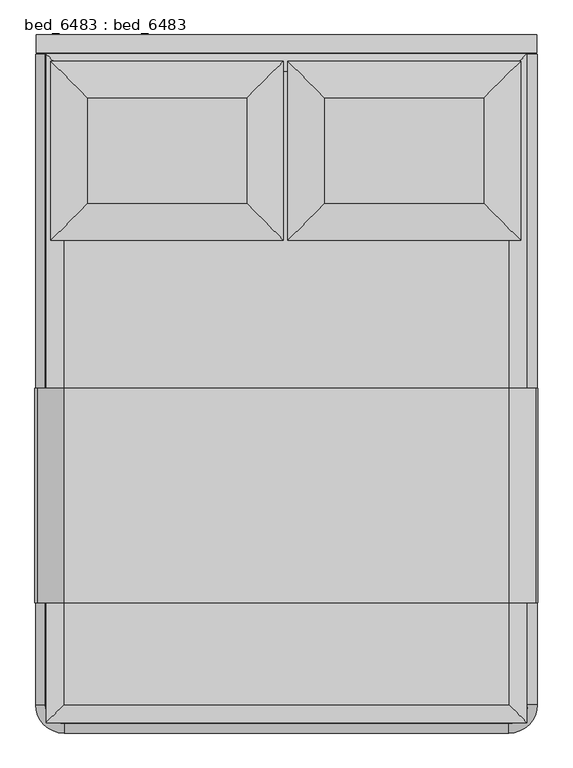
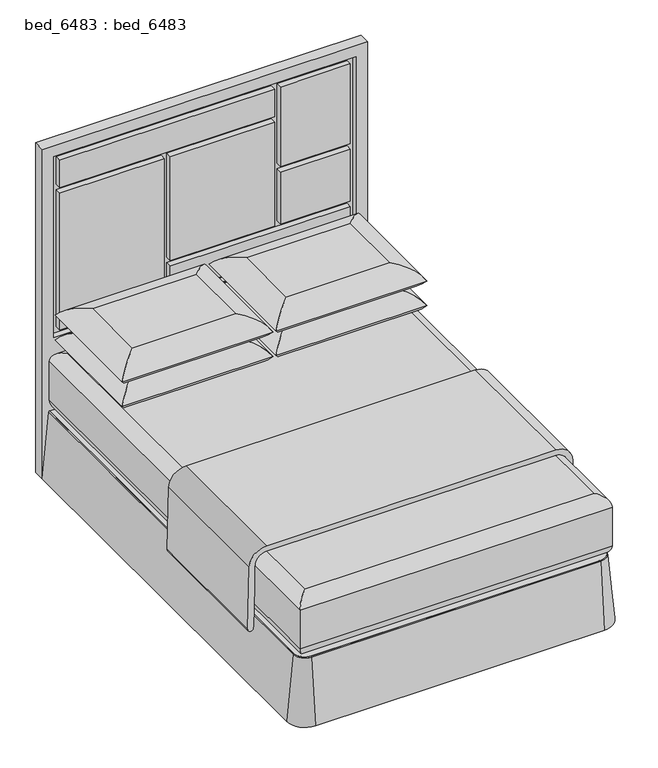
"""IFC4 building model written with IfcOpenShell, lengths in millimetres: proxy geometry, bed_6483 : bed_6483."""

from ifc_helpers import new_model, si_unit, point, frame, frame_2d, origin, place, context, project, spatial, polyline, circle_curve, ellipse_curve, trimmed, segment, composite_curve, outline, extrude, faceted_brep, source, transform, mapped, element, save
from ifc_brep_helpers import plane_surface, cylinder_surface, revolved_surface, advanced_brep


def bed_6483_bed_6483_9f93eb2d(model_context):
    return source(origin(), model_context, "Body", "SolidModel", [
        extrude(outline(composite_curve([segment(trimmed(circle_curve(frame_2d((494.8890898, 953.2998059)), 50.8), [point((494.8890898, 1004.0998059))], [point((545.6890898, 953.2998059))], False, "CARTESIAN"), True, "CONTINUOUS"), segment(polyline([(545.6890898, 953.2998059), (545.6890898, -843.7501941)]), True, "CONTINUOUS"), segment(trimmed(circle_curve(frame_2d((494.8890898, -843.7501941)), 50.8), [point((545.6890898, -843.7501941))], [point((494.8890898, -894.5501941))], False, "CARTESIAN"), True, "CONTINUOUS"), segment(polyline([(494.8890898, -894.5501941), (-768.7609102, -894.5501941)]), True, "CONTINUOUS"), segment(trimmed(circle_curve(frame_2d((-768.7609102, -843.7501941)), 50.8), [point((-768.7609102, -894.5501941))], [point((-819.5609102, -843.7501941))], False, "CARTESIAN"), True, "CONTINUOUS"), segment(polyline([(-819.5609102, -843.7501941), (-819.5609102, 953.2998059)]), True, "CONTINUOUS"), segment(trimmed(circle_curve(frame_2d((-768.7609102, 953.2998059)), 50.8), [point((-819.5609102, 953.2998059))], [point((-768.7609102, 1004.0998059))], False, "CARTESIAN"), True, "CONTINUOUS"), segment(polyline([(-768.7609102, 1004.0998059), (494.8890898, 1004.0998059)]), True, "CONTINUOUS")], self_intersect=False)), frame((0.0, 0.0, 152.4), z_axis=(0.0, 0.0, 1.0), x_axis=(1.0, 0.0, 0.0)), (0.0, 0.0, 1.0), 152.4),
        advanced_brep(
        [(-822.7359102, 1007.2748059, 149.225), (-822.7359102, 1007.2748059, 200.025), (-819.5609102, 1007.2748059, 200.025), (-819.5609102, 1007.2748059, 152.4), (-771.9359102, 1007.2748059, 152.4), (-771.9359102, 1007.2748059, 149.225), (-822.7359102, -843.7501941, 149.225), (-822.7359102, -843.7501941, 200.025), (-768.7609102, -897.7251941, 200.025), (494.8890898, -897.7251941, 200.025), (548.8640898, -843.7501941, 200.025), (548.8640898, 1007.2748059, 200.025), (545.6890898, 1007.2748059, 200.025), (545.6890898, -843.7501941, 200.025), (494.8890898, -894.5501941, 200.025), (-768.7609102, -894.5501941, 200.025), (-819.5609102, -843.7501941, 200.025), (-819.5609102, -843.7501941, 152.4), (-768.7609102, -894.5501941, 152.4), (494.8890898, -894.5501941, 152.4), (545.6890898, -843.7501941, 152.4), (545.6890898, 1007.2748059, 152.4), (498.0640898, 1007.2748059, 152.4), (498.0640898, -843.7501941, 152.4), (494.8890898, -846.9251941, 152.4), (-768.7609102, -846.9251941, 152.4), (-771.9359102, -843.7501941, 152.4), (-771.9359102, -843.7501941, 149.225), (-768.7609102, -846.9251941, 149.225), (494.8890898, -846.9251941, 149.225), (498.0640898, -843.7501941, 149.225), (498.0640898, 1007.2748059, 149.225), (548.8640898, 1007.2748059, 149.225), (548.8640898, -843.7501941, 149.225), (494.8890898, -897.7251941, 149.225), (-768.7609102, -897.7251941, 149.225)],
        [
            (0, 1),
            (1, 2),
            (2, 3),
            (3, 4),
            (4, 5),
            (5, 0),
            (0, 6),
            (6, 7),
            (7, 1),
            (7, 8, circle_curve(frame((-768.7609102, -843.7501941, 200.025), z_axis=(0.0, 0.0, 1.0), x_axis=(-1.0, 0.0, 0.0)), 53.975)),
            (8, 9),
            (9, 10, circle_curve(frame((494.8890898, -843.7501941, 200.025), z_axis=(0.0, 0.0, 1.0), x_axis=(0.0, -1.0, 0.0)), 53.975)),
            (10, 11),
            (11, 12),
            (12, 13),
            (13, 14, circle_curve(frame((494.8890898, -843.7501941, 200.025), z_axis=(0.0, 0.0, -1.0), x_axis=(0.0, -1.0, 0.0)), 50.8)),
            (14, 15),
            (15, 16, circle_curve(frame((-768.7609102, -843.7501941, 200.025), z_axis=(0.0, 0.0, -1.0), x_axis=(-1.0, 0.0, 0.0)), 50.8)),
            (16, 2),
            (16, 17),
            (17, 3),
            (17, 18, circle_curve(frame((-768.7609102, -843.7501941, 152.4), z_axis=(0.0, 0.0, 1.0), x_axis=(-1.0, 0.0, 0.0)), 50.8)),
            (18, 19),
            (19, 20, circle_curve(frame((494.8890898, -843.7501941, 152.4), z_axis=(0.0, 0.0, 1.0), x_axis=(0.0, -1.0, 0.0)), 50.8)),
            (20, 21),
            (21, 22),
            (22, 23),
            (23, 24, circle_curve(frame((494.8890898, -843.7501941, 152.4), z_axis=(0.0, 0.0, -1.0), x_axis=(0.0, -1.0, 0.0)), 3.175)),
            (24, 25),
            (25, 26, circle_curve(frame((-768.7609102, -843.7501941, 152.4), z_axis=(0.0, 0.0, -1.0), x_axis=(-1.0, 0.0, 0.0)), 3.175)),
            (26, 4),
            (26, 27),
            (27, 5),
            (27, 28, circle_curve(frame((-768.7609102, -843.7501941, 149.225), z_axis=(0.0, 0.0, 1.0), x_axis=(-1.0, 0.0, 0.0)), 3.175)),
            (28, 29),
            (29, 30, circle_curve(frame((494.8890898, -843.7501941, 149.225), z_axis=(0.0, 0.0, 1.0), x_axis=(0.0, -1.0, 0.0)), 3.175)),
            (30, 31),
            (31, 32),
            (32, 33),
            (33, 34, circle_curve(frame((494.8890898, -843.7501941, 149.225), z_axis=(0.0, 0.0, -1.0), x_axis=(0.0, -1.0, 0.0)), 53.975)),
            (34, 35),
            (35, 6, circle_curve(frame((-768.7609102, -843.7501941, 149.225), z_axis=(0.0, 0.0, -1.0), x_axis=(-1.0, 0.0, 0.0)), 53.975)),
            (35, 8),
            (15, 18),
            (25, 28),
            (34, 9),
            (14, 19),
            (24, 29),
            (33, 10),
            (13, 20),
            (23, 30),
            (31, 22),
            (21, 12),
            (11, 32),
        ],
        [
            plane_surface(frame((-822.7359102, 1007.2748059, 0.0), z_axis=(0.0, 1.0, 0.0), x_axis=(0.0, 0.0, 1.0))),
            plane_surface(frame((-822.7359102, 1007.2748059, 149.225), z_axis=(-1.0, 0.0, 0.0), x_axis=(0.0, -1.0, 0.0))),
            plane_surface(frame((-822.7359102, 1007.2748059, 200.025), z_axis=(0.0, 0.0, 1.0), x_axis=(0.0, -1.0, 0.0))),
            plane_surface(frame((-819.5609102, 1007.2748059, 200.025), z_axis=(1.0, 0.0, 0.0), x_axis=(0.0, -1.0, 0.0))),
            plane_surface(frame((-819.5609102, 1007.2748059, 152.4), z_axis=(0.0, 0.0, 1.0), x_axis=(0.0, -1.0, 0.0))),
            plane_surface(frame((-771.9359102, 1007.2748059, 152.4), z_axis=(1.0, 0.0, 0.0), x_axis=(0.0, -1.0, 0.0))),
            plane_surface(frame((-771.9359102, 1007.2748059, 149.225), z_axis=(0.0, 0.0, -1.0), x_axis=(0.0, -1.0, 0.0))),
            cylinder_surface(frame((-768.7609102, -843.7501941, 0.0), z_axis=(0.0, 0.0, 1.0), x_axis=(-1.0, 0.0, 0.0)), 53.975),
            revolved_surface(polyline([(-819.5609102, -843.7501941, 200.025), (-819.5609102, -843.7501941, 152.4)]), (-768.7609102, -843.7501941, 0.0), (0.0, 0.0, 1.0)),
            revolved_surface(polyline([(-771.9359102, -843.7501941, 152.4), (-771.9359102, -843.7501941, 149.225)]), (-768.7609102, -843.7501941, 0.0), (0.0, 0.0, 1.0)),
            plane_surface(frame((-768.7609102, -897.7251941, 149.225), z_axis=(0.0, -1.0, 0.0), x_axis=(1.0, 0.0, 0.0))),
            plane_surface(frame((-768.7609102, -894.5501941, 200.025), z_axis=(0.0, 1.0, 0.0), x_axis=(1.0, 0.0, 0.0))),
            plane_surface(frame((-768.7609102, -846.9251941, 152.4), z_axis=(0.0, 1.0, 0.0), x_axis=(1.0, 0.0, 0.0))),
            cylinder_surface(frame((494.8890898, -843.7501941, 0.0), z_axis=(0.0, 0.0, 1.0), x_axis=(0.0, -1.0, 0.0)), 53.975),
            revolved_surface(polyline([(494.8890898, -894.5501941, 200.025), (494.8890898, -894.5501941, 152.4)]), (494.8890898, -843.7501941, 0.0), (0.0, 0.0, 1.0)),
            revolved_surface(polyline([(494.8890898, -846.9251941, 152.4), (494.8890898, -846.9251941, 149.225)]), (494.8890898, -843.7501941, 0.0), (0.0, 0.0, 1.0)),
            plane_surface(frame((548.8640898, 1007.2748059, 0.0), z_axis=(0.0, 1.0, 0.0), x_axis=(0.0, 0.0, 1.0))),
            plane_surface(frame((548.8640898, -843.7501941, 149.225), z_axis=(1.0, 0.0, 0.0), x_axis=(0.0, 1.0, 0.0))),
            plane_surface(frame((545.6890898, -843.7501941, 200.025), z_axis=(-1.0, 0.0, 0.0), x_axis=(0.0, 1.0, 0.0))),
            plane_surface(frame((498.0640898, -843.7501941, 152.4), z_axis=(-1.0, 0.0, 0.0), x_axis=(0.0, 1.0, 0.0))),
        ],
        [
            (0, [[1, 2, 3, 4, 5, 6]]),
            (1, [[-1, 7, 8, 9]]),
            (2, [[-2, -9, 10, 11, 12, 13, 14, 15, 16, 17, 18, 19]]),
            (3, [[-3, -19, 20, 21]]),
            (4, [[-4, -21, 22, 23, 24, 25, 26, 27, 28, 29, 30, 31]]),
            (5, [[-5, -31, 32, 33]]),
            (6, [[-6, -33, 34, 35, 36, 37, 38, 39, 40, 41, 42, -7]]),
            (7, [[-10, -8, -42, 43]]),
            (8, [[-22, -20, -18, 44]]),
            (9, [[-34, -32, -30, 45]]),
            (10, [[-43, -41, 46, -11]]),
            (11, [[-44, -17, 47, -23]]),
            (12, [[-45, -29, 48, -35]]),
            (13, [[-12, -46, -40, 49]]),
            (14, [[-24, -47, -16, 50]]),
            (15, [[-36, -48, -28, 51]]),
            (16, [[-38, 52, -26, 53, -14, 54]]),
            (17, [[-49, -39, -54, -13]]),
            (18, [[-50, -15, -53, -25]]),
            (19, [[-51, -27, -52, -37]]),
        ],
    ),
        advanced_brep(
        [(-847.9072605, 1004.0998059, 2.4389304), (-849.5017215, 1004.0998059, 2.4389304), (-821.334659, 1004.0998059, 302.8875968), (-817.4912932, 1004.0998059, 306.3875), (-782.9739951, 1004.0998059, 306.3875), (-782.9739951, 1004.0998059, 304.8), (-819.5609102, 1004.0998059, 304.8), (-847.9072605, -843.7501941, 2.4389304), (-768.7609102, -922.8965443, 2.4389304), (494.8890898, -922.8965443, 2.4389304), (574.0354401, -843.7501941, 2.4389304), (574.0354401, 1004.0998059, 2.4389304), (575.6299011, 1004.0998059, 2.4389304), (575.6299011, -843.7501941, 2.4389304), (494.8890898, -924.4910054, 2.4389304), (-768.7609102, -924.4910054, 2.4389304), (-849.5017215, -843.7501941, 2.4389304), (-821.334659, -843.7501941, 302.8875968), (-817.4912932, -843.7501941, 306.3875), (-768.7609102, -892.480577, 306.3875), (494.8890898, -892.480577, 306.3875), (543.6194728, -843.7501941, 306.3875), (543.6194728, 1004.0998059, 306.3875), (509.1021747, 1004.0998059, 306.3875), (509.1021747, -843.7501941, 306.3875), (494.8890898, -857.9632789, 306.3875), (-768.7609102, -857.9632789, 306.3875), (-782.9739951, -843.7501941, 306.3875), (-782.9739951, -843.7501941, 304.8), (-768.7609102, -857.9632789, 304.8), (494.8890898, -857.9632789, 304.8), (509.1021747, -843.7501941, 304.8), (509.1021747, 1004.0998059, 304.8), (545.6890898, 1004.0998059, 304.8), (545.6890898, -843.7501941, 304.8), (494.8890898, -894.5501941, 304.8), (-768.7609102, -894.5501941, 304.8), (-819.5609102, -843.7501941, 304.8), (-768.7609102, -896.3239429, 302.8875968), (494.8890898, -896.3239429, 302.8875968), (547.4628387, -843.7501941, 302.8875968), (547.4628387, 1004.0998059, 302.8875968)],
        [
            (0, 1),
            (1, 2),
            (2, 3, circle_curve(frame((-817.4912932, 1004.0998059, 302.5272813), z_axis=(0.0, 1.0, 0.0), x_axis=(1.0, 0.0, 0.0)), 3.8602187)),
            (3, 4),
            (4, 5),
            (5, 6),
            (6, 0),
            (0, 7),
            (7, 8, circle_curve(frame((-768.7609102, -843.7501941, 2.4389304), z_axis=(0.0, 0.0, 1.0), x_axis=(-1.0, 0.0, 0.0)), 79.1463503)),
            (8, 9),
            (9, 10, circle_curve(frame((494.8890898, -843.7501941, 2.4389304), z_axis=(0.0, 0.0, 1.0), x_axis=(0.0, -1.0, 0.0)), 79.1463503)),
            (10, 11),
            (11, 12),
            (12, 13),
            (13, 14, circle_curve(frame((494.8890898, -843.7501941, 2.4389304), z_axis=(0.0, 0.0, -1.0), x_axis=(0.0, -1.0, 0.0)), 80.7408113)),
            (14, 15),
            (15, 16, circle_curve(frame((-768.7609102, -843.7501941, 2.4389304), z_axis=(0.0, 0.0, -1.0), x_axis=(-1.0, 0.0, 0.0)), 80.7408113)),
            (16, 1),
            (16, 17),
            (17, 2),
            (17, 18, circle_curve(frame((-817.4912932, -843.7501941, 302.5272813), z_axis=(0.0, 1.0, 0.0), x_axis=(1.0, 0.0, 0.0)), 3.8602187)),
            (18, 3),
            (18, 19, circle_curve(frame((-768.7609102, -843.7501941, 306.3875), z_axis=(0.0, 0.0, 1.0), x_axis=(-1.0, 0.0, 0.0)), 48.730383)),
            (19, 20),
            (20, 21, circle_curve(frame((494.8890898, -843.7501941, 306.3875), z_axis=(0.0, 0.0, 1.0), x_axis=(0.0, -1.0, 0.0)), 48.730383)),
            (21, 22),
            (22, 23),
            (23, 24),
            (24, 25, circle_curve(frame((494.8890898, -843.7501941, 306.3875), z_axis=(0.0, 0.0, -1.0), x_axis=(0.0, -1.0, 0.0)), 14.2130849)),
            (25, 26),
            (26, 27, circle_curve(frame((-768.7609102, -843.7501941, 306.3875), z_axis=(0.0, 0.0, -1.0), x_axis=(-1.0, 0.0, 0.0)), 14.2130849)),
            (27, 4),
            (27, 28),
            (28, 5),
            (28, 29, circle_curve(frame((-768.7609102, -843.7501941, 304.8), z_axis=(0.0, 0.0, 1.0), x_axis=(-1.0, 0.0, 0.0)), 14.2130849)),
            (29, 30),
            (30, 31, circle_curve(frame((494.8890898, -843.7501941, 304.8), z_axis=(0.0, 0.0, 1.0), x_axis=(0.0, -1.0, 0.0)), 14.2130849)),
            (31, 32),
            (32, 33),
            (33, 34),
            (34, 35, circle_curve(frame((494.8890898, -843.7501941, 304.8), z_axis=(0.0, 0.0, -1.0), x_axis=(0.0, -1.0, 0.0)), 50.8)),
            (35, 36),
            (36, 37, circle_curve(frame((-768.7609102, -843.7501941, 304.8), z_axis=(0.0, 0.0, -1.0), x_axis=(-1.0, 0.0, 0.0)), 50.8)),
            (37, 6),
            (37, 7),
            (15, 38),
            (38, 17, circle_curve(frame((-768.7609102, -843.7501941, 302.8875968), z_axis=(0.0, 0.0, -1.0), x_axis=(-1.0, 0.0, 0.0)), 52.5737489)),
            (38, 19, circle_curve(frame((-768.7609102, -892.480577, 302.5272813), z_axis=(-1.0, 0.0, 0.0), x_axis=(0.0, 1.0, 0.0)), 3.8602187)),
            (26, 29),
            (36, 8),
            (14, 39),
            (39, 38),
            (39, 20, circle_curve(frame((494.8890898, -892.480577, 302.5272813), z_axis=(-1.0, 0.0, 0.0), x_axis=(0.0, 1.0, 0.0)), 3.8602187)),
            (25, 30),
            (35, 9),
            (13, 40),
            (40, 39, circle_curve(frame((494.8890898, -843.7501941, 302.8875968), z_axis=(0.0, 0.0, -1.0), x_axis=(0.0, -1.0, 0.0)), 52.5737489)),
            (40, 21, circle_curve(frame((543.6194728, -843.7501941, 302.5272813), z_axis=(0.0, -1.0, 0.0), x_axis=(-1.0, 0.0, 0.0)), 3.8602187)),
            (24, 31),
            (34, 10),
            (11, 33),
            (32, 23),
            (22, 41, circle_curve(frame((543.6194728, 1004.0998059, 302.5272813), z_axis=(0.0, 1.0, 0.0), x_axis=(-1.0, 0.0, 0.0)), 3.8602187)),
            (41, 12),
            (41, 40),
        ],
        [
            plane_surface(frame((-819.5609102, 1004.0998059, 304.8), z_axis=(0.0, 1.0, 0.0), x_axis=(0.0, 0.0, 1.0))),
            plane_surface(frame((-847.9072605, 1004.0998059, 2.4389304), z_axis=(0.0, 0.0, -1.0), x_axis=(0.0, -1.0, 0.0))),
            plane_surface(frame((-849.5017215, 1004.0998059, 2.4389304), z_axis=(-0.9956342260592882, 0.0, 0.09334070869305766), x_axis=(0.0, -1.0, 0.0))),
            cylinder_surface(frame((-817.4912932, 1004.0998059, 302.5272813), z_axis=(0.0, 1.0, 0.0), x_axis=(1.0, 0.0, 0.0)), 3.8602187),
            plane_surface(frame((-817.4912932, 1004.0998059, 306.3875), z_axis=(0.0, 0.0, 1.0), x_axis=(0.0, -1.0, 0.0))),
            plane_surface(frame((-782.9739951, 1004.0998059, 306.3875), z_axis=(1.0, 0.0, 0.0), x_axis=(0.0, -1.0, 0.0))),
            plane_surface(frame((-782.9739951, 1004.0998059, 304.8), z_axis=(0.0, 0.0, -1.0), x_axis=(0.0, -1.0, 0.0))),
            plane_surface(frame((-819.5609102, 1004.0998059, 304.8), z_axis=(0.9956342260592882, 0.0, -0.09334070869305766), x_axis=(0.0, -1.0, 0.0))),
            revolved_surface(polyline([(-849.5017215, -843.7501941, 2.4389304), (-821.334659, -843.7501941, 302.8875968)]), (-768.7609102, -843.7501941, 304.8), (0.0, 0.0, 1.0)),
            revolved_surface(trimmed(ellipse_curve(frame((-817.4912932, -843.7501941, 302.5272813), z_axis=(0.0, 1.0, 0.0), x_axis=(1.0, 0.0, 0.0)), 3.8602187, 3.8602187), [point((-821.334659, -843.7501941, 302.8875968))], [point((-817.4912932, -843.7501941, 306.3875))], True, "CARTESIAN"), (-768.7609102, -843.7501941, 304.8), (0.0, 0.0, 1.0)),
            revolved_surface(polyline([(-782.9739951, -843.7501941, 306.3875), (-782.9739951, -843.7501941, 304.8)]), (-768.7609102, -843.7501941, 304.8), (0.0, 0.0, 1.0)),
            revolved_surface(polyline([(-819.5609102, -843.7501941, 304.8), (-847.9072605, -843.7501941, 2.4389304)]), (-768.7609102, -843.7501941, 304.8), (0.0, 0.0, 1.0)),
            plane_surface(frame((-768.7609102, -924.4910054, 2.4389304), z_axis=(0.0, -0.9956342260592882, 0.09334070869305766), x_axis=(1.0, 0.0, 0.0))),
            cylinder_surface(frame((-768.7609102, -892.480577, 302.5272813), z_axis=(-1.0, 0.0, 0.0), x_axis=(0.0, 1.0, 0.0)), 3.8602187),
            plane_surface(frame((-768.7609102, -857.9632789, 306.3875), z_axis=(0.0, 1.0, 0.0), x_axis=(1.0, 0.0, 0.0))),
            plane_surface(frame((-768.7609102, -894.5501941, 304.8), z_axis=(0.0, 0.9956342260592882, -0.09334070869305766), x_axis=(1.0, 0.0, 0.0))),
            revolved_surface(polyline([(494.8890898, -924.4910054, 2.4389304), (494.8890898, -896.3239429, 302.8875968)]), (494.8890898, -843.7501941, 304.8), (0.0, 0.0, 1.0)),
            revolved_surface(trimmed(ellipse_curve(frame((494.8890898, -892.480577, 302.5272813), z_axis=(-1.0, 0.0, 0.0), x_axis=(0.0, 1.0, 0.0)), 3.8602187, 3.8602187), [point((494.8890898, -896.3239429, 302.8875968))], [point((494.8890898, -892.480577, 306.3875))], True, "CARTESIAN"), (494.8890898, -843.7501941, 304.8), (0.0, 0.0, 1.0)),
            revolved_surface(polyline([(494.8890898, -857.963279, 306.3875), (494.8890898, -857.963279, 304.8)]), (494.8890898, -843.7501941, 304.8), (0.0, 0.0, 1.0)),
            revolved_surface(polyline([(494.8890898, -894.5501941, 304.8), (494.8890898, -922.8965443, 2.4389304)]), (494.8890898, -843.7501941, 304.8), (0.0, 0.0, 1.0)),
            plane_surface(frame((545.6890898, 1004.0998059, 304.8), z_axis=(0.0, 1.0, 0.0), x_axis=(0.0, 0.0, 1.0))),
            plane_surface(frame((575.6299011, -843.7501941, 2.4389304), z_axis=(0.9956342260592882, 0.0, 0.09334070869305766), x_axis=(0.0, 1.0, 0.0))),
            cylinder_surface(frame((543.6194728, -843.7501941, 302.5272813), z_axis=(0.0, -1.0, 0.0), x_axis=(-1.0, 0.0, 0.0)), 3.8602187),
            plane_surface(frame((509.1021747, -843.7501941, 306.3875), z_axis=(-1.0, 0.0, 0.0), x_axis=(0.0, 1.0, 0.0))),
            plane_surface(frame((545.6890898, -843.7501941, 304.8), z_axis=(-0.9956342260592882, 0.0, -0.09334070869305766), x_axis=(0.0, 1.0, 0.0))),
        ],
        [
            (0, [[1, 2, 3, 4, 5, 6, 7]]),
            (1, [[-1, 8, 9, 10, 11, 12, 13, 14, 15, 16, 17, 18]]),
            (2, [[-2, -18, 19, 20]]),
            (3, [[-3, -20, 21, 22]]),
            (4, [[-4, -22, 23, 24, 25, 26, 27, 28, 29, 30, 31, 32]]),
            (5, [[-5, -32, 33, 34]]),
            (6, [[-6, -34, 35, 36, 37, 38, 39, 40, 41, 42, 43, 44]]),
            (7, [[-7, -44, 45, -8]]),
            (8, [[-17, 46, 47, -19]]),
            (9, [[-21, -47, 48, -23]]),
            (10, [[-31, 49, -35, -33]]),
            (11, [[-9, -45, -43, 50]]),
            (12, [[-16, 51, 52, -46]]),
            (13, [[-24, -48, -52, 53]]),
            (14, [[-30, 54, -36, -49]]),
            (15, [[-10, -50, -42, 55]]),
            (16, [[-15, 56, 57, -51]]),
            (17, [[-25, -53, -57, 58]]),
            (18, [[-29, 59, -37, -54]]),
            (19, [[-11, -55, -41, 60]]),
            (20, [[-13, 61, -39, 62, -27, 63, 64]]),
            (21, [[-14, -64, 65, -56]]),
            (22, [[-26, -58, -65, -63]]),
            (23, [[-28, -62, -38, -59]]),
            (24, [[-12, -60, -40, -61]]),
        ],
    ),
        advanced_brep(
        [(-768.7609102, -843.7501941, 585.7875), (494.8890898, -843.7501941, 585.7875), (494.8890898, 470.9562082, 585.7875), (494.8890898, 953.2998059, 585.7875), (-136.9359102, 953.2998059, 585.7875), (-141.1561538, 953.2998059, 585.7875), (-768.7609102, 953.2998059, 585.7875), (-768.7609102, 470.9562082, 585.7875), (494.8890898, -843.7501941, 306.3875), (-768.7609102, -843.7501941, 306.3875), (-768.7609102, 953.2998059, 306.3875), (494.8890898, 953.2998059, 306.3875), (545.6890898, 1004.0998059, 534.9875), (545.6890898, 1004.0998059, 357.1875), (-819.5609102, 1004.0998059, 357.1875), (-819.5609102, 1004.0998059, 534.9875), (-819.5609102, -894.5501941, 357.1875), (-819.5609102, -894.5501941, 534.9875), (545.6890898, -894.5501941, 357.1875), (545.6890898, -894.5501941, 534.9875)],
        [
            (0, 1),
            (1, 2),
            (2, 3),
            (3, 4),
            (4, 5),
            (5, 6),
            (6, 7),
            (7, 0),
            (8, 9),
            (9, 10),
            (10, 11),
            (11, 8),
            (12, 13),
            (13, 14),
            (14, 15),
            (15, 12),
            (14, 16),
            (16, 17),
            (17, 15),
            (16, 18),
            (18, 19),
            (19, 17),
            (12, 19),
            (18, 13),
            (19, 1, ellipse_curve(frame((494.8890898, -843.7501941, 534.9875), z_axis=(-0.7071067811865475, -0.7071067811865475, 0.0), x_axis=(0.7071067811865476, -0.7071067811865474, 0.0)), 71.842049, 50.8)),
            (0, 17, ellipse_curve(frame((-768.7609102, -843.7501941, 534.9875), z_axis=(0.7071067811865475, -0.7071067811865475, 0.0), x_axis=(0.7071067811865476, 0.7071067811865474, 0.0)), 71.842049, 50.8)),
            (8, 18, ellipse_curve(frame((494.8890898, -843.7501941, 357.1875), z_axis=(-0.7071067811865475, -0.7071067811865475, 0.0), x_axis=(0.7071067811865476, -0.7071067811865474, 0.0)), 71.842049, 50.8)),
            (16, 9, ellipse_curve(frame((-768.7609102, -843.7501941, 357.1875), z_axis=(0.7071067811865475, -0.7071067811865475, 0.0), x_axis=(0.7071067811865476, 0.7071067811865474, 0.0)), 71.842049, 50.8)),
            (12, 3, ellipse_curve(frame((494.8890898, 953.2998059, 534.9875), z_axis=(0.7071067811865475, -0.7071067811865475, 0.0), x_axis=(0.7071067811865474, 0.7071067811865476, 0.0)), 71.842049, 50.8)),
            (11, 13, ellipse_curve(frame((494.8890898, 953.2998059, 357.1875), z_axis=(0.7071067811865475, -0.7071067811865475, 0.0), x_axis=(0.7071067811865474, 0.7071067811865476, 0.0)), 71.842049, 50.8)),
            (15, 6, ellipse_curve(frame((-768.7609102, 953.2998059, 534.9875), z_axis=(0.7071067811865475, 0.7071067811865475, 0.0), x_axis=(-0.7071067811865476, 0.7071067811865474, 0.0)), 71.842049, 50.8)),
            (10, 14, ellipse_curve(frame((-768.7609102, 953.2998059, 357.1875), z_axis=(0.7071067811865475, 0.7071067811865475, 0.0), x_axis=(-0.7071067811865476, 0.7071067811865474, 0.0)), 71.842049, 50.8)),
        ],
        [
            plane_surface(frame((-819.5609102, 1004.0998059, 585.7875), z_axis=(0.0, 0.0, 1.0), x_axis=(-1.0, 0.0, 0.0))),
            plane_surface(frame((-819.5609102, 1004.0998059, 306.3875), z_axis=(0.0, 0.0, -1.0), x_axis=(1.0, 0.0, 0.0))),
            plane_surface(frame((545.6890898, 1004.0998059, 585.7875), z_axis=(0.0, 1.0, 0.0), x_axis=(0.0, 0.0, -1.0))),
            plane_surface(frame((-819.5609102, 1004.0998059, 585.7875), z_axis=(-1.0, 0.0, 0.0), x_axis=(0.0, 0.0, -1.0))),
            plane_surface(frame((-819.5609102, -894.5501941, 585.7875), z_axis=(0.0, -1.0, 0.0), x_axis=(0.0, 0.0, -1.0))),
            plane_surface(frame((545.6890898, -894.5501941, 585.7875), z_axis=(1.0, 0.0, 0.0), x_axis=(0.0, 0.0, -1.0))),
            cylinder_surface(frame((-819.5609102, -843.7501941, 534.9875), z_axis=(1.0, 0.0, 0.0), x_axis=(0.0, 1.0, 0.0)), 50.8),
            cylinder_surface(frame((-819.5609102, -843.7501941, 357.1875), z_axis=(1.0, 0.0, 0.0), x_axis=(0.0, 1.0, 0.0)), 50.8),
            cylinder_surface(frame((494.8890898, -894.5501941, 534.9875), z_axis=(0.0, 1.0, 0.0), x_axis=(-1.0, 0.0, 0.0)), 50.8),
            cylinder_surface(frame((494.8890898, -894.5501941, 357.1875), z_axis=(0.0, 1.0, 0.0), x_axis=(-1.0, 0.0, 0.0)), 50.8),
            cylinder_surface(frame((545.6890898, 953.2998059, 534.9875), z_axis=(-1.0, 0.0, 0.0), x_axis=(0.0, -1.0, 0.0)), 50.8),
            cylinder_surface(frame((545.6890898, 953.2998059, 357.1875), z_axis=(-1.0, 0.0, 0.0), x_axis=(0.0, -1.0, 0.0)), 50.8),
            cylinder_surface(frame((-768.7609102, 1004.0998059, 534.9875), z_axis=(0.0, -1.0, 0.0), x_axis=(1.0, 0.0, 0.0)), 50.8),
            cylinder_surface(frame((-768.7609102, 1004.0998059, 357.1875), z_axis=(0.0, -1.0, 0.0), x_axis=(1.0, 0.0, 0.0)), 50.8),
        ],
        [
            (0, [[1, 2, 3, 4, 5, 6, 7, 8]]),
            (1, [[9, 10, 11, 12]]),
            (2, [[13, 14, 15, 16]]),
            (3, [[-15, 17, 18, 19]]),
            (4, [[-18, 20, 21, 22]]),
            (5, [[-13, 23, -21, 24]]),
            (6, [[25, -1, 26, -22]]),
            (7, [[27, -20, 28, -9]]),
            (8, [[-25, -23, 29, -3, -2]]),
            (9, [[-27, -12, 30, -24]]),
            (10, [[-29, -16, 31, -6, -5, -4]]),
            (11, [[-30, -11, 32, -14]]),
            (12, [[-26, -8, -7, -31, -19]]),
            (13, [[-28, -17, -32, -10]]),
        ],
    ),
        faceted_brep([(-848.1359102, 1007.2748059, 1524.0), (-848.1359102, 1007.2748059, 0.0), (-746.5359102, 1007.2748059, 0.0), (-746.5359102, 1007.2748059, 127.0), (472.6640898, 1007.2748059, 127.0), (472.6640898, 1007.2748059, 0.0), (574.2640898, 1007.2748059, 0.0), (574.2640898, 1007.2748059, 1524.0), (-797.3359102, 1007.2748059, 1473.2), (523.4640898, 1007.2748059, 1473.2), (523.4640898, 1007.2748059, 636.5875), (-797.3359102, 1007.2748059, 636.5875), (167.8640898, 1007.2748059, 1320.8), (167.8640898, 1007.2748059, 1447.8), (-771.9359102, 1007.2748059, 1447.8), (-771.9359102, 1007.2748059, 1320.8), (-314.7359102, 1007.2748059, 1295.4), (-771.9359102, 1007.2748059, 1295.4), (-771.9359102, 1007.2748059, 661.9875), (-314.7359102, 1007.2748059, 661.9875), (193.2640898, 1007.2748059, 1080.29375), (498.0640898, 1007.2748059, 1080.29375), (498.0640898, 1007.2748059, 1447.8), (193.2640898, 1007.2748059, 1447.8), (498.0640898, 1007.2748059, 1054.89375), (193.2640898, 1007.2748059, 1054.89375), (193.2640898, 1007.2748059, 814.3875), (498.0640898, 1007.2748059, 814.3875), (-289.3359102, 1007.2748059, 1295.4), (-289.3359102, 1007.2748059, 814.3875), (167.8640898, 1007.2748059, 814.3875), (167.8640898, 1007.2748059, 1295.4), (498.0640898, 1007.2748059, 661.9875), (498.0640898, 1007.2748059, 788.9875), (-289.3359102, 1007.2748059, 788.9875), (-289.3359102, 1007.2748059, 661.9875), (-848.1359102, 1058.0748059, 1524.0), (574.2640898, 1058.0748059, 1524.0), (574.2640898, 1058.0748059, 0.0), (472.6640898, 1058.0748059, 0.0), (472.6640898, 1058.0748059, 127.0), (-746.5359102, 1058.0748059, 127.0), (-746.5359102, 1058.0748059, 0.0), (-848.1359102, 1058.0748059, 0.0), (523.4640898, 1032.6748059, 1473.2), (-797.3359102, 1032.6748059, 1473.2), (-797.3359102, 1032.6748059, 636.5875), (523.4640898, 1032.6748059, 636.5875), (167.8640898, 1032.6748059, 1447.8), (167.8640898, 1032.6748059, 1320.8), (-771.9359102, 1032.6748059, 1320.8), (-771.9359102, 1032.6748059, 1447.8), (-771.9359102, 1032.6748059, 1295.4), (-314.7359102, 1032.6748059, 1295.4), (-314.7359102, 1032.6748059, 661.9875), (-771.9359102, 1032.6748059, 661.9875), (498.0640898, 1032.6748059, 1080.29375), (193.2640898, 1032.6748059, 1080.29375), (193.2640898, 1032.6748059, 1447.8), (498.0640898, 1032.6748059, 1447.8), (193.2640898, 1032.6748059, 1054.89375), (498.0640898, 1032.6748059, 1054.89375), (498.0640898, 1032.6748059, 814.3875), (193.2640898, 1032.6748059, 814.3875), (-289.3359102, 1032.6748059, 814.3875), (-289.3359102, 1032.6748059, 1295.4), (167.8640898, 1032.6748059, 1295.4), (167.8640898, 1032.6748059, 814.3875), (498.0640898, 1032.6748059, 788.9875), (498.0640898, 1032.6748059, 661.9875), (-289.3359102, 1032.6748059, 661.9875), (-289.3359102, 1032.6748059, 788.9875)], [[[0, 1, 2, 3, 4, 5, 6, 7], [8, 9, 10, 11]], [[12, 13, 14, 15]], [[16, 17, 18, 19]], [[20, 21, 22, 23]], [[24, 25, 26, 27]], [[28, 29, 30, 31]], [[32, 33, 34, 35]], [[36, 37, 38, 39, 40, 41, 42, 43]], [[1, 0, 36, 43]], [[2, 1, 43, 42]], [[3, 2, 42, 41]], [[4, 3, 41, 40]], [[5, 4, 40, 39]], [[6, 5, 39, 38]], [[7, 6, 38, 37]], [[0, 7, 37, 36]], [[44, 45, 46, 47], [48, 49, 50, 51], [52, 53, 54, 55], [56, 57, 58, 59], [60, 61, 62, 63], [64, 65, 66, 67], [68, 69, 70, 71]], [[45, 44, 9, 8]], [[46, 45, 8, 11]], [[47, 46, 11, 10]], [[44, 47, 10, 9]], [[49, 48, 13, 12]], [[50, 49, 12, 15]], [[51, 50, 15, 14]], [[48, 51, 14, 13]], [[53, 52, 17, 16]], [[54, 53, 16, 19]], [[55, 54, 19, 18]], [[52, 55, 18, 17]], [[57, 56, 21, 20]], [[58, 57, 20, 23]], [[59, 58, 23, 22]], [[56, 59, 22, 21]], [[61, 60, 25, 24]], [[62, 61, 24, 27]], [[63, 62, 27, 26]], [[60, 63, 26, 25]], [[65, 64, 29, 28]], [[66, 65, 28, 31]], [[67, 66, 31, 30]], [[64, 67, 30, 29]], [[69, 68, 33, 32]], [[70, 69, 32, 35]], [[71, 70, 35, 34]], [[68, 71, 34, 33]]]),
        advanced_brep(
        [(-28.0171423, 579.8749761, 700.0875), (423.0250783, 579.8749761, 700.0875), (423.0250783, 878.5171967, 700.0875), (-28.0171423, 878.5171967, 700.0875), (423.0250783, 579.8749761, 585.7875), (-28.0171423, 579.8749761, 585.7875), (-28.0171423, 878.5171967, 585.7875), (423.0250783, 878.5171967, 585.7875), (-132.696032, 475.1960864, 642.9375), (527.703968, 475.1960864, 642.9375), (527.703968, 983.1960864, 642.9375), (-132.696032, 983.1960864, 642.9375)],
        [
            (0, 1),
            (1, 2),
            (2, 3),
            (3, 0),
            (4, 5),
            (5, 6),
            (6, 7),
            (7, 4),
            (8, 9),
            (9, 1, ellipse_curve(frame((423.0250783, 579.8749761, 575.6448714), z_axis=(-0.7071067811865474, -0.7071067811865476, 0.0), x_axis=(0.7071067811865477, -0.7071067811865474, 0.0)), 175.9884531, 124.4426286)),
            (0, 8, ellipse_curve(frame((-28.0171423, 579.8749761, 575.6448714), z_axis=(0.7071067811865478, -0.7071067811865471, 0.0), x_axis=(0.7071067811865472, 0.7071067811865477, 0.0)), 175.9884531, 124.4426286)),
            (8, 5, ellipse_curve(frame((-28.0171423, 579.8749761, 710.2301286), z_axis=(0.7071067811865478, -0.7071067811865471, 0.0), x_axis=(0.7071067811865472, 0.7071067811865477, 0.0)), 175.9884531, 124.4426286)),
            (4, 9, ellipse_curve(frame((423.0250783, 579.8749761, 710.2301286), z_axis=(-0.7071067811865474, -0.7071067811865476, 0.0), x_axis=(0.7071067811865477, -0.7071067811865474, 0.0)), 175.9884531, 124.4426286)),
            (9, 10),
            (10, 2, ellipse_curve(frame((423.0250783, 878.5171967, 575.6448714), z_axis=(0.7071067811865476, -0.7071067811865474, 0.0), x_axis=(0.7071067811865474, 0.7071067811865478, 0.0)), 175.9884531, 124.4426286)),
            (7, 10, ellipse_curve(frame((423.0250783, 878.5171967, 710.2301286), z_axis=(0.7071067811865476, -0.7071067811865474, 0.0), x_axis=(0.7071067811865474, 0.7071067811865478, 0.0)), 175.9884531, 124.4426286)),
            (10, 11),
            (11, 3, ellipse_curve(frame((-28.0171423, 878.5171967, 575.6448714), z_axis=(0.7071067811865471, 0.7071067811865477, 0.0), x_axis=(-0.7071067811865481, 0.707106781186547, 0.0)), 175.9884531, 124.4426286)),
            (6, 11, ellipse_curve(frame((-28.0171423, 878.5171967, 710.2301286), z_axis=(0.7071067811865471, 0.7071067811865477, 0.0), x_axis=(-0.7071067811865481, 0.707106781186547, 0.0)), 175.9884531, 124.4426286)),
            (11, 8),
        ],
        [
            plane_surface(frame((-132.696032, 983.1960864, 700.0875), z_axis=(0.0, 0.0, 1.0), x_axis=(-1.0, 0.0, 0.0))),
            plane_surface(frame((-132.696032, 983.1960864, 585.7875), z_axis=(0.0, 0.0, -1.0), x_axis=(1.0, 0.0, 0.0))),
            cylinder_surface(frame((-132.696032, 579.8749761, 575.6448714), z_axis=(1.0, 0.0, 0.0), x_axis=(0.0, 1.0, 0.0)), 124.4426286),
            cylinder_surface(frame((-132.696032, 579.8749761, 710.2301286), z_axis=(1.0, 0.0, 0.0), x_axis=(0.0, 1.0, 0.0)), 124.4426286),
            cylinder_surface(frame((423.0250783, 475.1960864, 575.6448714), z_axis=(0.0, 1.0, 0.0), x_axis=(-1.0, 0.0, 0.0)), 124.4426286),
            cylinder_surface(frame((423.0250783, 475.1960864, 710.2301286), z_axis=(0.0, 1.0, 0.0), x_axis=(-1.0, 0.0, 0.0)), 124.4426286),
            cylinder_surface(frame((527.703968, 878.5171967, 575.6448714), z_axis=(-1.0, 0.0, 0.0), x_axis=(0.0, -1.0, 0.0)), 124.4426286),
            cylinder_surface(frame((527.703968, 878.5171967, 710.2301286), z_axis=(-1.0, 0.0, 0.0), x_axis=(0.0, -1.0, 0.0)), 124.4426286),
            cylinder_surface(frame((-28.0171423, 983.1960864, 575.6448714), z_axis=(0.0, -1.0, 0.0), x_axis=(1.0, 0.0, 0.0)), 124.4426286),
            cylinder_surface(frame((-28.0171423, 983.1960864, 710.2301286), z_axis=(0.0, -1.0, 0.0), x_axis=(1.0, 0.0, 0.0)), 124.4426286),
        ],
        [
            (0, [[1, 2, 3, 4]]),
            (1, [[5, 6, 7, 8]]),
            (2, [[9, 10, -1, 11]]),
            (3, [[-9, 12, -5, 13]]),
            (4, [[-10, 14, 15, -2]]),
            (5, [[-13, -8, 16, -14]]),
            (6, [[-15, 17, 18, -3]]),
            (7, [[-16, -7, 19, -17]]),
            (8, [[-11, -4, -18, 20]]),
            (9, [[-12, -20, -19, -6]]),
        ],
    ),
        advanced_brep(
        [(-701.1171423, 579.8749761, 700.0875), (-250.0749217, 579.8749761, 700.0875), (-250.0749217, 878.5171967, 700.0875), (-701.1171423, 878.5171967, 700.0875), (-250.0749217, 579.8749761, 585.7875), (-701.1171423, 579.8749761, 585.7875), (-701.1171423, 878.5171967, 585.7875), (-250.0749217, 878.5171967, 585.7875), (-805.796032, 475.1960864, 642.9375), (-145.396032, 475.1960864, 642.9375), (-145.396032, 983.1960864, 642.9375), (-805.796032, 983.1960864, 642.9375)],
        [
            (0, 1),
            (1, 2),
            (2, 3),
            (3, 0),
            (4, 5),
            (5, 6),
            (6, 7),
            (7, 4),
            (8, 9),
            (9, 1, ellipse_curve(frame((-250.0749217, 579.8749761, 575.6448714), z_axis=(-0.7071067811865475, -0.7071067811865475, 0.0), x_axis=(0.7071067811865476, -0.7071067811865475, 0.0)), 175.9884531, 124.4426286)),
            (0, 8, ellipse_curve(frame((-701.1171423, 579.8749761, 575.6448714), z_axis=(0.7071067811865477, -0.7071067811865472, 0.0), x_axis=(0.7071067811865475, 0.7071067811865475, 0.0)), 175.9884531, 124.4426286)),
            (8, 5, ellipse_curve(frame((-701.1171423, 579.8749761, 710.2301286), z_axis=(0.7071067811865477, -0.7071067811865472, 0.0), x_axis=(0.7071067811865475, 0.7071067811865475, 0.0)), 175.9884531, 124.4426286)),
            (4, 9, ellipse_curve(frame((-250.0749217, 579.8749761, 710.2301286), z_axis=(-0.7071067811865475, -0.7071067811865475, 0.0), x_axis=(0.7071067811865476, -0.7071067811865475, 0.0)), 175.9884531, 124.4426286)),
            (9, 10),
            (10, 2, ellipse_curve(frame((-250.0749217, 878.5171967, 575.6448714), z_axis=(0.7071067811865475, -0.7071067811865475, 0.0), x_axis=(0.7071067811865472, 0.7071067811865477, 0.0)), 175.9884531, 124.4426286)),
            (7, 10, ellipse_curve(frame((-250.0749217, 878.5171967, 710.2301286), z_axis=(0.7071067811865475, -0.7071067811865475, 0.0), x_axis=(0.7071067811865472, 0.7071067811865477, 0.0)), 175.9884531, 124.4426286)),
            (10, 11),
            (11, 3, ellipse_curve(frame((-701.1171423, 878.5171967, 575.6448714), z_axis=(0.7071067811865472, 0.7071067811865477, 0.0), x_axis=(-0.7071067811865478, 0.7071067811865472, 0.0)), 175.9884531, 124.4426286)),
            (6, 11, ellipse_curve(frame((-701.1171423, 878.5171967, 710.2301286), z_axis=(0.7071067811865472, 0.7071067811865477, 0.0), x_axis=(-0.7071067811865478, 0.7071067811865472, 0.0)), 175.9884531, 124.4426286)),
            (11, 8),
        ],
        [
            plane_surface(frame((-805.796032, 983.1960864, 700.0875), z_axis=(0.0, 0.0, 1.0), x_axis=(-1.0, 0.0, 0.0))),
            plane_surface(frame((-805.796032, 983.1960864, 585.7875), z_axis=(0.0, 0.0, -1.0), x_axis=(1.0, 0.0, 0.0))),
            cylinder_surface(frame((-805.796032, 579.8749761, 575.6448714), z_axis=(1.0, 0.0, 0.0), x_axis=(0.0, 1.0, 0.0)), 124.4426286),
            cylinder_surface(frame((-805.796032, 579.8749761, 710.2301286), z_axis=(1.0, 0.0, 0.0), x_axis=(0.0, 1.0, 0.0)), 124.4426286),
            cylinder_surface(frame((-250.0749217, 475.1960864, 575.6448714), z_axis=(0.0, 1.0, 0.0), x_axis=(-1.0, 0.0, 0.0)), 124.4426286),
            cylinder_surface(frame((-250.0749217, 475.1960864, 710.2301286), z_axis=(0.0, 1.0, 0.0), x_axis=(-1.0, 0.0, 0.0)), 124.4426286),
            cylinder_surface(frame((-145.396032, 878.5171967, 575.6448714), z_axis=(-1.0, 0.0, 0.0), x_axis=(0.0, -1.0, 0.0)), 124.4426286),
            cylinder_surface(frame((-145.396032, 878.5171967, 710.2301286), z_axis=(-1.0, 0.0, 0.0), x_axis=(0.0, -1.0, 0.0)), 124.4426286),
            cylinder_surface(frame((-701.1171423, 983.1960864, 575.6448714), z_axis=(0.0, -1.0, 0.0), x_axis=(1.0, 0.0, 0.0)), 124.4426286),
            cylinder_surface(frame((-701.1171423, 983.1960864, 710.2301286), z_axis=(0.0, -1.0, 0.0), x_axis=(1.0, 0.0, 0.0)), 124.4426286),
        ],
        [
            (0, [[1, 2, 3, 4]]),
            (1, [[5, 6, 7, 8]]),
            (2, [[9, 10, -1, 11]]),
            (3, [[-9, 12, -5, 13]]),
            (4, [[-10, 14, 15, -2]]),
            (5, [[-13, -8, 16, -14]]),
            (6, [[-15, 17, 18, -3]]),
            (7, [[-16, -7, 19, -17]]),
            (8, [[-11, -4, -18, 20]]),
            (9, [[-12, -20, -19, -6]]),
        ],
    ),
        advanced_brep(
        [(-28.0171423, 579.8749761, 814.3875), (423.0250783, 579.8749761, 814.3875), (423.0250783, 878.5171967, 814.3875), (-28.0171423, 878.5171967, 814.3875), (423.0250783, 579.8749761, 700.0875), (-28.0171423, 579.8749761, 700.0875), (-28.0171423, 878.5171967, 700.0875), (423.0250783, 878.5171967, 700.0875), (-132.696032, 475.1960864, 757.2375), (527.703968, 475.1960864, 757.2375), (527.703968, 983.1960864, 757.2375), (-132.696032, 983.1960864, 757.2375)],
        [
            (0, 1),
            (1, 2),
            (2, 3),
            (3, 0),
            (4, 5),
            (5, 6),
            (6, 7),
            (7, 4),
            (8, 9),
            (9, 1, ellipse_curve(frame((423.0250783, 579.8749761, 689.9448714), z_axis=(-0.7071067811865474, -0.7071067811865476, 0.0), x_axis=(0.7071067811865477, -0.7071067811865474, 0.0)), 175.9884531, 124.4426286)),
            (0, 8, ellipse_curve(frame((-28.0171423, 579.8749761, 689.9448714), z_axis=(0.7071067811865478, -0.7071067811865471, 0.0), x_axis=(0.7071067811865472, 0.7071067811865477, 0.0)), 175.9884531, 124.4426286)),
            (8, 5, ellipse_curve(frame((-28.0171423, 579.8749761, 824.5301286), z_axis=(0.7071067811865478, -0.7071067811865471, 0.0), x_axis=(0.7071067811865472, 0.7071067811865477, 0.0)), 175.9884531, 124.4426286)),
            (4, 9, ellipse_curve(frame((423.0250783, 579.8749761, 824.5301286), z_axis=(-0.7071067811865474, -0.7071067811865476, 0.0), x_axis=(0.7071067811865477, -0.7071067811865474, 0.0)), 175.9884531, 124.4426286)),
            (9, 10),
            (10, 2, ellipse_curve(frame((423.0250783, 878.5171967, 689.9448714), z_axis=(0.7071067811865476, -0.7071067811865474, 0.0), x_axis=(0.7071067811865474, 0.7071067811865478, 0.0)), 175.9884531, 124.4426286)),
            (7, 10, ellipse_curve(frame((423.0250783, 878.5171967, 824.5301286), z_axis=(0.7071067811865476, -0.7071067811865474, 0.0), x_axis=(0.7071067811865474, 0.7071067811865478, 0.0)), 175.9884531, 124.4426286)),
            (10, 11),
            (11, 3, ellipse_curve(frame((-28.0171423, 878.5171967, 689.9448714), z_axis=(0.7071067811865471, 0.7071067811865477, 0.0), x_axis=(-0.7071067811865481, 0.707106781186547, 0.0)), 175.9884531, 124.4426286)),
            (6, 11, ellipse_curve(frame((-28.0171423, 878.5171967, 824.5301286), z_axis=(0.7071067811865471, 0.7071067811865477, 0.0), x_axis=(-0.7071067811865481, 0.707106781186547, 0.0)), 175.9884531, 124.4426286)),
            (11, 8),
        ],
        [
            plane_surface(frame((-132.696032, 983.1960864, 814.3875), z_axis=(0.0, 0.0, 1.0), x_axis=(-1.0, 0.0, 0.0))),
            plane_surface(frame((-132.696032, 983.1960864, 700.0875), z_axis=(0.0, 0.0, -1.0), x_axis=(1.0, 0.0, 0.0))),
            cylinder_surface(frame((-132.696032, 579.8749761, 689.9448714), z_axis=(1.0, 0.0, 0.0), x_axis=(0.0, 1.0, 0.0)), 124.4426286),
            cylinder_surface(frame((-132.696032, 579.8749761, 824.5301286), z_axis=(1.0, 0.0, 0.0), x_axis=(0.0, 1.0, 0.0)), 124.4426286),
            cylinder_surface(frame((423.0250783, 475.1960864, 689.9448714), z_axis=(0.0, 1.0, 0.0), x_axis=(-1.0, 0.0, 0.0)), 124.4426286),
            cylinder_surface(frame((423.0250783, 475.1960864, 824.5301286), z_axis=(0.0, 1.0, 0.0), x_axis=(-1.0, 0.0, 0.0)), 124.4426286),
            cylinder_surface(frame((527.703968, 878.5171967, 689.9448714), z_axis=(-1.0, 0.0, 0.0), x_axis=(0.0, -1.0, 0.0)), 124.4426286),
            cylinder_surface(frame((527.703968, 878.5171967, 824.5301286), z_axis=(-1.0, 0.0, 0.0), x_axis=(0.0, -1.0, 0.0)), 124.4426286),
            cylinder_surface(frame((-28.0171423, 983.1960864, 689.9448714), z_axis=(0.0, -1.0, 0.0), x_axis=(1.0, 0.0, 0.0)), 124.4426286),
            cylinder_surface(frame((-28.0171423, 983.1960864, 824.5301286), z_axis=(0.0, -1.0, 0.0), x_axis=(1.0, 0.0, 0.0)), 124.4426286),
        ],
        [
            (0, [[1, 2, 3, 4]]),
            (1, [[5, 6, 7, 8]]),
            (2, [[9, 10, -1, 11]]),
            (3, [[-9, 12, -5, 13]]),
            (4, [[-10, 14, 15, -2]]),
            (5, [[-13, -8, 16, -14]]),
            (6, [[-15, 17, 18, -3]]),
            (7, [[-16, -7, 19, -17]]),
            (8, [[-11, -4, -18, 20]]),
            (9, [[-12, -20, -19, -6]]),
        ],
    ),
        advanced_brep(
        [(-701.1171423, 579.8749761, 814.3875), (-250.0749217, 579.8749761, 814.3875), (-250.0749217, 878.5171967, 814.3875), (-701.1171423, 878.5171967, 814.3875), (-250.0749217, 579.8749761, 700.0875), (-701.1171423, 579.8749761, 700.0875), (-701.1171423, 878.5171967, 700.0875), (-250.0749217, 878.5171967, 700.0875), (-805.796032, 475.1960864, 757.2375), (-145.396032, 475.1960864, 757.2375), (-145.396032, 983.1960864, 757.2375), (-805.796032, 983.1960864, 757.2375)],
        [
            (0, 1),
            (1, 2),
            (2, 3),
            (3, 0),
            (4, 5),
            (5, 6),
            (6, 7),
            (7, 4),
            (8, 9),
            (9, 1, ellipse_curve(frame((-250.0749217, 579.8749761, 689.9448714), z_axis=(-0.7071067811865475, -0.7071067811865475, 0.0), x_axis=(0.7071067811865477, -0.7071067811865472, 0.0)), 175.9884531, 124.4426286)),
            (0, 8, ellipse_curve(frame((-701.1171423, 579.8749761, 689.9448714), z_axis=(0.7071067811865476, -0.7071067811865475, 0.0), x_axis=(0.7071067811865475, 0.7071067811865476, 0.0)), 175.9884531, 124.4426286)),
            (8, 5, ellipse_curve(frame((-701.1171423, 579.8749761, 824.5301286), z_axis=(0.7071067811865476, -0.7071067811865475, 0.0), x_axis=(0.7071067811865475, 0.7071067811865476, 0.0)), 175.9884531, 124.4426286)),
            (4, 9, ellipse_curve(frame((-250.0749217, 579.8749761, 824.5301286), z_axis=(-0.7071067811865475, -0.7071067811865475, 0.0), x_axis=(0.7071067811865477, -0.7071067811865472, 0.0)), 175.9884531, 124.4426286)),
            (9, 10),
            (10, 2, ellipse_curve(frame((-250.0749217, 878.5171967, 689.9448714), z_axis=(0.7071067811865476, -0.7071067811865474, 0.0), x_axis=(0.7071067811865472, 0.7071067811865478, 0.0)), 175.9884531, 124.4426286)),
            (7, 10, ellipse_curve(frame((-250.0749217, 878.5171967, 824.5301286), z_axis=(0.7071067811865476, -0.7071067811865474, 0.0), x_axis=(0.7071067811865472, 0.7071067811865478, 0.0)), 175.9884531, 124.4426286)),
            (10, 11),
            (11, 3, ellipse_curve(frame((-701.1171423, 878.5171967, 689.9448714), z_axis=(0.7071067811865474, 0.7071067811865476, 0.0), x_axis=(-0.7071067811865478, 0.7071067811865472, 0.0)), 175.9884531, 124.4426286)),
            (6, 11, ellipse_curve(frame((-701.1171423, 878.5171967, 824.5301286), z_axis=(0.7071067811865474, 0.7071067811865476, 0.0), x_axis=(-0.7071067811865478, 0.7071067811865472, 0.0)), 175.9884531, 124.4426286)),
            (11, 8),
        ],
        [
            plane_surface(frame((-805.796032, 983.1960864, 814.3875), z_axis=(0.0, 0.0, 1.0), x_axis=(-1.0, 0.0, 0.0))),
            plane_surface(frame((-805.796032, 983.1960864, 700.0875), z_axis=(0.0, 0.0, -1.0), x_axis=(1.0, 0.0, 0.0))),
            cylinder_surface(frame((-805.796032, 579.8749761, 689.9448714), z_axis=(1.0, 0.0, 0.0), x_axis=(0.0, 1.0, 0.0)), 124.4426286),
            cylinder_surface(frame((-805.796032, 579.8749761, 824.5301286), z_axis=(1.0, 0.0, 0.0), x_axis=(0.0, 1.0, 0.0)), 124.4426286),
            cylinder_surface(frame((-250.0749217, 475.1960864, 689.9448714), z_axis=(0.0, 1.0, 0.0), x_axis=(-1.0, 0.0, 0.0)), 124.4426286),
            cylinder_surface(frame((-250.0749217, 475.1960864, 824.5301286), z_axis=(0.0, 1.0, 0.0), x_axis=(-1.0, 0.0, 0.0)), 124.4426286),
            cylinder_surface(frame((-145.396032, 878.5171967, 689.9448714), z_axis=(-1.0, 0.0, 0.0), x_axis=(0.0, -1.0, 0.0)), 124.4426286),
            cylinder_surface(frame((-145.396032, 878.5171967, 824.5301286), z_axis=(-1.0, 0.0, 0.0), x_axis=(0.0, -1.0, 0.0)), 124.4426286),
            cylinder_surface(frame((-701.1171423, 983.1960864, 689.9448714), z_axis=(0.0, -1.0, 0.0), x_axis=(1.0, 0.0, 0.0)), 124.4426286),
            cylinder_surface(frame((-701.1171423, 983.1960864, 824.5301286), z_axis=(0.0, -1.0, 0.0), x_axis=(1.0, 0.0, 0.0)), 124.4426286),
        ],
        [
            (0, [[1, 2, 3, 4]]),
            (1, [[5, 6, 7, 8]]),
            (2, [[9, 10, -1, 11]]),
            (3, [[-9, 12, -5, 13]]),
            (4, [[-10, 14, 15, -2]]),
            (5, [[-13, -8, 16, -14]]),
            (6, [[-15, 17, 18, -3]]),
            (7, [[-16, -7, 19, -17]]),
            (8, [[-11, -4, -18, 20]]),
            (9, [[-12, -20, -19, -6]]),
        ],
    ),
        extrude(outline(composite_curve([segment(trimmed(circle_curve(frame_2d((536.1441512, -769.9175614)), 49.6301793), [point((536.1441512, -819.5477407))], [point((585.7743306, -769.9175614))], True, "CARTESIAN"), True, "CONTINUOUS"), segment(polyline([(585.7743306, -769.9175614), (585.7743306, 494.8890898)]), True, "CONTINUOUS"), segment(trimmed(circle_curve(frame_2d((534.9743306, 494.8890898)), 50.8), [point((585.7743306, 494.8890898))], [point((525.3316297, 544.7655203))], True, "CARTESIAN"), True, "CONTINUOUS"), segment(polyline([(525.3316297, 544.7655203), (253.2166596, 550.9628378)]), True, "CONTINUOUS"), segment(trimmed(circle_curve(frame_2d((253.2166596, 563.666131)), 12.7032932), [point((253.2166596, 550.9628378))], [point((253.2166596, 576.3694242))], False, "CARTESIAN"), True, "CONTINUOUS"), segment(polyline([(253.2166596, 576.3694242), (523.4634866, 570.214653)]), True, "CONTINUOUS"), segment(trimmed(circle_curve(frame_2d((534.9743306, 494.8890898)), 76.2), [point((523.4634866, 570.214653))], [point((611.1743306, 494.8890898))], False, "CARTESIAN"), True, "CONTINUOUS"), segment(polyline([(611.1743306, 494.8890898), (611.1743306, -769.9175614)]), True, "CONTINUOUS"), segment(trimmed(circle_curve(frame_2d((536.1441512, -769.9175614)), 75.0301793), [point((611.1743306, -769.9175614))], [point((536.463122, -844.9470627))], False, "CARTESIAN"), True, "CONTINUOUS"), segment(polyline([(536.463122, -844.9470627), (253.7949853, -851.3847247)]), True, "CONTINUOUS"), segment(trimmed(circle_curve(frame_2d((253.7949853, -838.6814315)), 12.7032932), [point((253.7949853, -851.3847247))], [point((253.7949853, -825.9781383))], False, "CARTESIAN"), True, "CONTINUOUS"), segment(polyline([(253.7949853, -825.9781383), (536.1441512, -819.5477407)]), True, "CONTINUOUS")], self_intersect=False)), frame((0.0, -554.8251941, 0.0), z_axis=(0.0, 1.0, 0.0), x_axis=(0.0, 0.0, 1.0)), (0.0, 0.0, 1.0), 609.6),
    ])


if __name__ == "__main__":
    model = new_model("IFC4")
    model_context = context("Model", 3, world=origin())
    ifc_project = project(units=[si_unit("LENGTHUNIT", "METRE", prefix="MILLI")], contexts=[model_context])
    site = spatial("IfcSite", under=ifc_project)
    building = spatial("IfcBuilding", under=site)
    placement = place(None, origin())
    bed_6483_bed_6483_shape = bed_6483_bed_6483_9f93eb2d(model_context)
    element("IfcBuildingElementProxy", 1, Name="bed_6483 : bed_6483", ObjectType="bed_6483 : bed_6483", at=placement, inside=building, context=model_context, shape_type="MappedRepresentation", body=[
        mapped(bed_6483_bed_6483_shape, transform((0.0, 0.0, 0.0), x_axis=(1.0, 0.0, 0.0), y_axis=(0.0, 1.0, 0.0), z_axis=(0.0, 0.0, 1.0))),
    ])
    save(model, "model.ifc")

# Revit data of these elements
# Type "bed_6483 : bed_6483"
#   wood = none
#   fabric 2 [instance default] = none
#   fabric [instance default] = none
#   Mirror = none
#   Default Elevation = 0
# Element 1 (IfcBuildingElementProxy, "bed_6483 : bed_6483")
#   Materials on its faces: "wood", "fabric", "fabric 2", "mirror", "chrome"
# Materials
#   "wood": class "Wood", colour RGB 71 38 7, transparency 0
#   "fabric": class "Fabric", colour RGB 56 56 56, transparency 0
#   "fabric 2": class "Fabric", colour RGB 64 0 0, transparency 0
#   "mirror": class "Glass", colour RGB 228 228 228, transparency 0.06
#   "chrome": class "Metal", colour RGB 244 244 244, transparency 0
